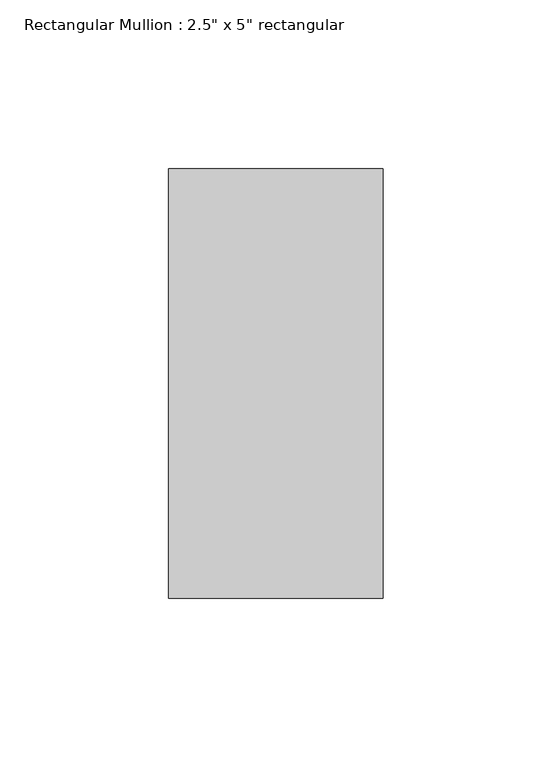
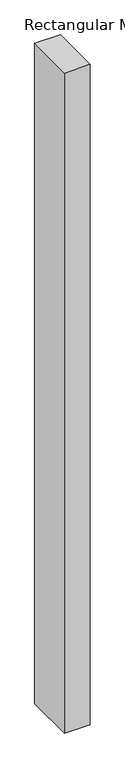
"""IFC4 building model written with IfcOpenShell, lengths in millimetres: member geometry."""

from ifc_helpers import new_model, si_unit, frame, origin, place, context, project, spatial, polyline, outline, extrude, source, transform, mapped, element, save


def member_b63e54e1(model_context):
    return source(origin(), model_context, "Body", "SweptSolid", [
        extrude(outline(polyline([(0.0, 63.5), (0.0, -63.5), (-63.5, -63.5), (-63.5, 63.5), (0.0, 63.5)])), frame((0.0, 0.0, -1718.7125392), z_axis=(0.0, 0.0, 1.0), x_axis=(1.0, 0.0, 0.0)), (0.0, 0.0, 1.0), 1718.7125392),
    ])


if __name__ == "__main__":
    model = new_model("IFC4")
    model_context = context("Model", 3, world=origin())
    ifc_project = project(units=[si_unit("LENGTHUNIT", "METRE", prefix="MILLI")], contexts=[model_context])
    site = spatial("IfcSite", under=ifc_project)
    building = spatial("IfcBuilding", under=site)
    placement = place(None, origin())
    member_shape = member_b63e54e1(model_context)
    element("IfcMember", 1, ObjectType="Rectangular Mullion : 2.5\" x 5\" rectangular", at=placement, inside=building, context=model_context, shape_type="MappedRepresentation", body=[
        mapped(member_shape, transform((0.0, 0.0, 0.0), x_axis=(1.0, 0.0, 0.0), y_axis=(0.0, 1.0, 0.0), z_axis=(0.0, 0.0, 1.0))),
    ])
    save(model, "model.ifc")

# Revit data of these elements
# Type "Rectangular Mullion : 2.5\" x 5\" rectangular"
#   built-in parameter 1007304 = 0.416667 (stored number, unit not read)
#   built-in parameter 1007301 = 0.104167 (stored number, unit not read)
#   built-in parameter 1007300 = 0.104167 (stored number, unit not read)
# Element 1 (IfcMember, "Rectangular Mullion : 2.5\" x 5\" rectangular")
#   Materials on its faces: "Aluminum"
# Materials
#   "Aluminum": class "Metal", colour RGB 247 247 247, transparency 0, Description = "Aluminum 6061", Cost = 0
